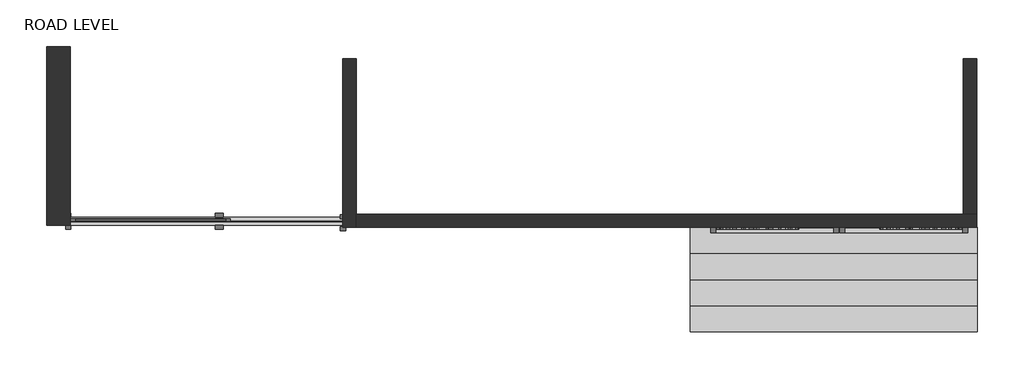
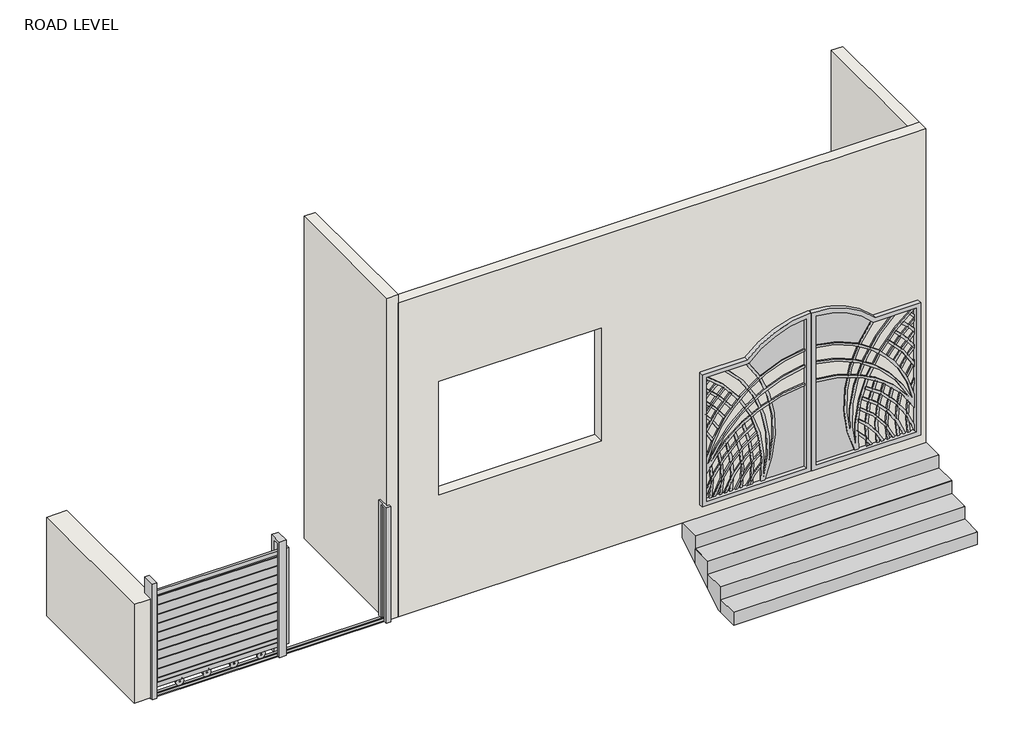
# One storey: 4 walls, 1 geographic element, 1 proxy, 1 stair flight.
"""IFC4 building model written with IfcOpenShell, lengths in millimetres."""

from ifc_helpers import new_model, si_unit, point, frame, frame_2d, origin, place, context, project, spatial, polyline, circle_curve, trimmed, segment, composite_curve, outline, extrude, faceted_brep, transform, mapped, element, save
from components import gate_7956_gate_7956_6bc30956

model = new_model("IFC4")

# Units and contexts
model_context = context("Model", 3, world=origin())
ifc_project = project(units=[si_unit("LENGTHUNIT", "METRE", prefix="MILLI")], contexts=[model_context])

# Site, building, storey
site = spatial("IfcSite", under=ifc_project)
building = spatial("IfcBuilding", under=site)
storey = spatial("IfcBuildingStorey", under=building, Name="ROAD LEVEL", Elevation=457.2)

# Proxy
placement = place(None, origin())
gate_7956_gate_7956_shape = gate_7956_gate_7956_6bc30956(model_context)
element("IfcBuildingElementProxy", 1, Name="gate_7956 : gate_7956", ObjectType="gate_7956 : gate_7956", at=placement, inside=storey, context=model_context, shape_type="MappedRepresentation", body=[
    mapped(gate_7956_gate_7956_shape, transform((8127.3305046, -8538.9053244, 1066.8), x_axis=(1.0, 0.0, 0.0), y_axis=(0.0, 1.0, 0.0), z_axis=(0.0, 0.0, 1.0))),
])

# Geographic element
element("IfcGeographicElement", 2, ObjectType="Sliding_Gate_17236 : Sliding_Gate_17236", at=placement, inside=storey, context=model_context, shape_type="SolidModel", body=[
    extrude(outline(polyline([(-8474.623372, 914.4), (-8443.6553244, 914.4), (-8443.6553244, 901.7), (-8519.8553244, 901.7), (-8519.8553244, 914.4), (-8489.076024, 914.4), (-8489.076024, 913.0780612), (-8474.623372, 913.0780612), (-8474.623372, 914.4)])), frame((742.1222446, 0.0, 0.0), z_axis=(1.0, 0.0, 0.0), x_axis=(0.0, 1.0, 0.0)), (0.0, 0.0, 1.0), 2649.5789518),
    faceted_brep([(792.9222446, -8405.5553244, 914.4), (792.9222446, -8443.6553244, 914.4), (788.1495839, -8443.6553244, 914.4), (788.1495839, -8405.5553244, 914.4), (792.9222446, -8443.6553244, 2260.6), (767.5222446, -8443.6553244, 2260.6), (767.5222446, -8443.6553244, 2089.1943747), (788.1495839, -8443.6553244, 2089.1943747), (767.5222446, -8519.8553244, 2260.6), (767.5222446, -8519.8553244, 2089.1943747), (792.9222446, -8519.8553244, 2260.6), (792.9222446, -8519.8553244, 914.4), (742.1222446, -8519.8553244, 914.4), (742.1222446, -8519.8553244, 2089.1943747), (742.1222446, -8557.9553244, 914.4), (792.9222446, -8557.9553244, 914.4), (792.9222446, -8557.9553244, 2286.0), (742.1222446, -8557.9553244, 2286.0), (742.1222446, -8405.5553244, 2286.0), (742.1222446, -8405.5553244, 2089.1943747), (792.9222446, -8405.5553244, 2286.0), (788.1495839, -8405.5553244, 2089.1943747)], [[[0, 1, 2, 3]], [[1, 4, 5, 6, 7, 2]], [[5, 8, 9, 6]], [[8, 10, 11, 12, 13, 9]], [[14, 15, 16, 17]], [[14, 17, 18, 19, 13, 12]], [[18, 20, 0, 3, 21, 19]], [[1, 0, 20, 16, 15, 11, 10, 4]], [[5, 4, 10, 8]], [[17, 16, 20, 18]], [[7, 21, 3, 2]], [[21, 7, 6, 9, 13, 19]], [[12, 11, 15, 14]]]),
    extrude(outline(polyline([(-8405.5553244, 2286.0), (-8405.5553244, 914.4), (-8443.6553244, 914.4), (-8443.6553244, 2247.9), (-8519.8553244, 2247.9), (-8519.8553244, 914.4), (-8557.9553244, 914.4), (-8557.9553244, 2286.0), (-8405.5553244, 2286.0)])), frame((2170.8722446, 0.0, 0.0), z_axis=(1.0, 0.0, 0.0), x_axis=(0.0, 1.0, 0.0)), (0.0, 0.0, 1.0), 76.2),
    extrude(outline(polyline([(2087.8280612, 2272.4722446), (2087.8280612, 837.3722446), (1033.7280612, 837.3722446), (1033.7280612, 2272.4722446), (2087.8280612, 2272.4722446)]), holes=[polyline([(2062.4280612, 862.7722446), (2062.4280612, 2247.0722446), (2056.0780612, 2247.0722446), (2056.0780612, 862.7722446), (2062.4280612, 862.7722446)]), polyline([(1954.4780612, 862.7722446), (1954.4780612, 2247.0722446), (1948.1280612, 2247.0722446), (1948.1280612, 862.7722446), (1954.4780612, 862.7722446)]), polyline([(1846.5280612, 862.7722446), (1846.5280612, 2247.0722446), (1840.1780612, 2247.0722446), (1840.1780612, 862.7722446), (1846.5280612, 862.7722446)]), polyline([(1738.5780612, 862.7722446), (1738.5780612, 2247.0722446), (1732.2280612, 2247.0722446), (1732.2280612, 862.7722446), (1738.5780612, 862.7722446)]), polyline([(1630.6280612, 862.7722446), (1630.6280612, 2247.0722446), (1624.2780612, 2247.0722446), (1624.2780612, 862.7722446), (1630.6280612, 862.7722446)]), polyline([(1522.6780612, 862.7722446), (1522.6780612, 2247.0722446), (1516.3280612, 2247.0722446), (1516.3280612, 862.7722446), (1522.6780612, 862.7722446)]), polyline([(1414.7280612, 862.7722446), (1414.7280612, 2247.0722446), (1408.3780612, 2247.0722446), (1408.3780612, 862.7722446), (1414.7280612, 862.7722446)]), polyline([(1306.7780612, 862.7722446), (1306.7780612, 2247.0722446), (1300.4280612, 2247.0722446), (1300.4280612, 862.7722446), (1306.7780612, 862.7722446)]), polyline([(1198.8280612, 862.7722446), (1198.8280612, 2247.0722446), (1192.4780612, 2247.0722446), (1192.4780612, 862.7722446), (1198.8280612, 862.7722446)]), polyline([(1090.8780612, 862.7722446), (1090.8780612, 2247.0722446), (1084.5280612, 2247.0722446), (1084.5280612, 862.7722446), (1090.8780612, 862.7722446)])]), frame((0.0, -8476.376024, 0.0), z_axis=(0.0, 1.0, 0.0), x_axis=(0.0, 0.0, 1.0)), (0.0, 0.0, 1.0), 12.7),
    extrude(outline(polyline([(2132.2780612, 2316.9222446), (2132.2780612, 792.9222446), (989.2780612, 792.9222446), (989.2780612, 2316.9222446), (2132.2780612, 2316.9222446)]), holes=[polyline([(2081.4780612, 843.7222446), (2081.4780612, 2266.1222446), (1040.0780612, 2266.1222446), (1040.0780612, 843.7222446), (2081.4780612, 843.7222446)])]), frame((0.0, -8482.726024, 0.0), z_axis=(0.0, 1.0, 0.0), x_axis=(0.0, 0.0, 1.0)), (0.0, 0.0, 1.0), 25.4),
    extrude(outline(composite_curve([segment(trimmed(circle_curve(frame_2d((957.5280612, 1402.5222446)), 44.45), [point((957.5280612, 1358.0722446))], [point((957.5280612, 1446.9722446))], False, "CARTESIAN"), True, "CONTINUOUS"), segment(trimmed(circle_curve(frame_2d((957.5280612, 1402.5222446)), 44.45), [point((957.5280612, 1446.9722446))], [point((957.5280612, 1358.0722446))], False, "CARTESIAN"), True, "CONTINUOUS")], self_intersect=False), holes=[composite_curve([segment(trimmed(circle_curve(frame_2d((957.5280612, 1402.5222446)), 6.35), [point((957.5280612, 1396.1722446))], [point((957.5280612, 1408.8722446))], True, "CARTESIAN"), True, "CONTINUOUS"), segment(trimmed(circle_curve(frame_2d((957.5280612, 1402.5222446)), 6.35), [point((957.5280612, 1408.8722446))], [point((957.5280612, 1396.1722446))], True, "CARTESIAN"), True, "CONTINUOUS")], self_intersect=False)]), frame((0.0, -8476.376024, 0.0), z_axis=(0.0, 1.0, 0.0), x_axis=(0.0, 0.0, 1.0)), (0.0, 0.0, 1.0), 12.7),
    extrude(outline(composite_curve([segment(trimmed(circle_curve(frame_2d((957.5280612, 2012.1222446)), 44.45), [point((957.5280612, 1967.6722446))], [point((957.5280612, 2056.5722446))], False, "CARTESIAN"), True, "CONTINUOUS"), segment(trimmed(circle_curve(frame_2d((957.5280612, 2012.1222446)), 44.45), [point((957.5280612, 2056.5722446))], [point((957.5280612, 1967.6722446))], False, "CARTESIAN"), True, "CONTINUOUS")], self_intersect=False), holes=[composite_curve([segment(trimmed(circle_curve(frame_2d((957.5280612, 2012.1222446)), 6.35), [point((957.5280612, 2005.7722446))], [point((957.5280612, 2018.4722446))], True, "CARTESIAN"), True, "CONTINUOUS"), segment(trimmed(circle_curve(frame_2d((957.5280612, 2012.1222446)), 6.35), [point((957.5280612, 2018.4722446))], [point((957.5280612, 2005.7722446))], True, "CARTESIAN"), True, "CONTINUOUS")], self_intersect=False)]), frame((0.0, -8476.376024, 0.0), z_axis=(0.0, 1.0, 0.0), x_axis=(0.0, 0.0, 1.0)), (0.0, 0.0, 1.0), 12.7),
    extrude(outline(composite_curve([segment(trimmed(circle_curve(frame_2d((957.5280612, 1707.3222446)), 44.45), [point((957.5280612, 1662.8722446))], [point((957.5280612, 1751.7722446))], False, "CARTESIAN"), True, "CONTINUOUS"), segment(trimmed(circle_curve(frame_2d((957.5280612, 1707.3222446)), 44.45), [point((957.5280612, 1751.7722446))], [point((957.5280612, 1662.8722446))], False, "CARTESIAN"), True, "CONTINUOUS")], self_intersect=False), holes=[composite_curve([segment(trimmed(circle_curve(frame_2d((957.5280612, 1707.3222446)), 6.35), [point((957.5280612, 1700.9722446))], [point((957.5280612, 1713.6722446))], True, "CARTESIAN"), True, "CONTINUOUS"), segment(trimmed(circle_curve(frame_2d((957.5280612, 1707.3222446)), 6.35), [point((957.5280612, 1713.6722446))], [point((957.5280612, 1700.9722446))], True, "CARTESIAN"), True, "CONTINUOUS")], self_intersect=False)]), frame((0.0, -8476.376024, 0.0), z_axis=(0.0, 1.0, 0.0), x_axis=(0.0, 0.0, 1.0)), (0.0, 0.0, 1.0), 12.7),
    extrude(outline(composite_curve([segment(trimmed(circle_curve(frame_2d((957.5280612, 1097.7222446)), 44.45), [point((957.5280612, 1053.2722446))], [point((957.5280612, 1142.1722446))], False, "CARTESIAN"), True, "CONTINUOUS"), segment(trimmed(circle_curve(frame_2d((957.5280612, 1097.7222446)), 44.45), [point((957.5280612, 1142.1722446))], [point((957.5280612, 1053.2722446))], False, "CARTESIAN"), True, "CONTINUOUS")], self_intersect=False), holes=[composite_curve([segment(trimmed(circle_curve(frame_2d((957.5280612, 1097.7222446)), 6.35), [point((957.5280612, 1091.3722446))], [point((957.5280612, 1104.0722446))], True, "CARTESIAN"), True, "CONTINUOUS"), segment(trimmed(circle_curve(frame_2d((957.5280612, 1097.7222446)), 6.35), [point((957.5280612, 1104.0722446))], [point((957.5280612, 1091.3722446))], True, "CARTESIAN"), True, "CONTINUOUS")], self_intersect=False)]), frame((0.0, -8476.376024, 0.0), z_axis=(0.0, 1.0, 0.0), x_axis=(0.0, 0.0, 1.0)), (0.0, 0.0, 1.0), 12.7),
    faceted_brep([(3366.3011964, -8418.2553244, 914.4), (3417.1011964, -8418.2553244, 914.4), (3417.1011964, -8570.6553244, 914.4), (3366.3011964, -8570.6553244, 914.4), (3366.3011964, -8532.5553244, 914.4), (3391.7011964, -8532.5553244, 914.4), (3391.7011964, -8456.3553244, 914.4), (3366.3011964, -8456.3553244, 914.4), (3391.7011964, -8456.3553244, 2260.6), (3366.3011964, -8456.3553244, 2260.6), (3391.7011964, -8532.5553244, 2260.6), (3366.3011964, -8532.5553244, 2260.6), (3366.3011964, -8570.6553244, 2286.0), (3417.1011964, -8570.6553244, 2286.0), (3417.1011964, -8418.2553244, 2286.0), (3366.3011964, -8418.2553244, 2286.0)], [[[0, 1, 2, 3, 4, 5, 6, 7]], [[6, 8, 9, 7]], [[5, 10, 8, 6]], [[4, 11, 10, 5]], [[12, 3, 2, 13]], [[13, 2, 1, 14]], [[14, 1, 0, 15]], [[11, 4, 3, 12, 15, 0, 7, 9]], [[9, 8, 10, 11]], [[12, 13, 14, 15]]]),
])

# Stair flight
element("IfcStairFlight", 3, ObjectType="1mm_Tread-150mm_Depth", at=placement, inside=storey, context=model_context, shape_type="SolidModel", body=[
    faceted_brep([(6712.3831457, -9288.9053244, 456.2), (6712.3831457, -9538.9053244, 456.2), (9454.4805046, -9538.9053244, 456.2), (9454.4805046, -9288.9053244, 456.2), (6712.3831457, -9288.9053244, 304.8), (6712.3831457, -9538.9053244, 304.8), (9454.4805046, -9538.9053244, 304.8), (9454.4805046, -9288.9053244, 304.8), (6712.3831457, -9038.9053244, 608.6), (6712.3831457, -9288.9053244, 608.6), (9454.4805046, -9288.9053244, 608.6), (9454.4805046, -9038.9053244, 608.6), (6712.3831457, -9038.9053244, 432.9262296), (6712.3831457, -9249.0861473, 304.8), (9454.4805046, -9249.0861473, 304.8), (9454.4805046, -9038.9053244, 432.9262296), (6712.3831457, -8788.9053244, 585.3262296), (6712.3831457, -8538.9053244, 737.7262296), (9454.4805046, -8538.9053244, 737.7262296), (9454.4805046, -8788.9053244, 585.3262296), (6712.3831457, -8788.9053244, 761.0), (6712.3831457, -9038.9053244, 761.0), (9454.4805046, -9038.9053244, 761.0), (9454.4805046, -8788.9053244, 761.0), (6712.3831457, -8538.9053244, 913.4), (6712.3831457, -8788.9053244, 913.4), (9454.4805046, -8788.9053244, 913.4), (9454.4805046, -8538.9053244, 913.4)], [[[0, 1, 2, 3]], [[1, 0, 4, 5]], [[2, 1, 5, 6]], [[3, 2, 6, 7]], [[8, 9, 10, 11]], [[4, 0, 9, 8, 12, 13]], [[0, 3, 10, 9]], [[3, 7, 14, 15, 11, 10]], [[5, 4, 13, 14, 7, 6]], [[14, 13, 12, 16, 17, 18, 19, 15]], [[20, 21, 22, 23]], [[21, 20, 16, 12, 8]], [[8, 11, 22, 21]], [[23, 22, 11, 15, 19]], [[24, 25, 26, 27]], [[25, 24, 17, 16, 20]], [[20, 23, 26, 25]], [[27, 26, 23, 19, 18]], [[24, 27, 18, 17]]]),
    extrude(outline(polyline([(6712.3831457, -9288.9053244), (9454.4805046, -9288.9053244), (9454.4805046, -9538.9053244), (6712.3831457, -9538.9053244), (6712.3831457, -9288.9053244)])), frame((0.0, 0.0, 456.2), z_axis=(0.0, 0.0, 1.0), x_axis=(1.0, 0.0, 0.0)), (0.0, 0.0, 1.0), 1.0),
    extrude(outline(polyline([(6712.3831457, -9038.9053244), (9454.4805046, -9038.9053244), (9454.4805046, -9288.9053244), (6712.3831457, -9288.9053244), (6712.3831457, -9038.9053244)])), frame((0.0, 0.0, 608.6), z_axis=(0.0, 0.0, 1.0), x_axis=(1.0, 0.0, 0.0)), (0.0, 0.0, 1.0), 1.0),
    extrude(outline(polyline([(6712.3831457, -8788.9053244), (9454.4805046, -8788.9053244), (9454.4805046, -9038.9053244), (6712.3831457, -9038.9053244), (6712.3831457, -8788.9053244)])), frame((0.0, 0.0, 761.0), z_axis=(0.0, 0.0, 1.0), x_axis=(1.0, 0.0, 0.0)), (0.0, 0.0, 1.0), 1.0),
    extrude(outline(polyline([(6712.3831457, -8538.9053244), (9454.4805046, -8538.9053244), (9454.4805046, -8788.9053244), (6712.3831457, -8788.9053244), (6712.3831457, -8538.9053244)])), frame((0.0, 0.0, 913.4), z_axis=(0.0, 0.0, 1.0), x_axis=(1.0, 0.0, 0.0)), (0.0, 0.0, 1.0), 1.0),
])

# Walls
element("IfcWall", 4, ObjectType="5\"", at=placement, inside=storey, context=model_context, shape_type="Brep", body=[
    faceted_brep([(3517.0722446, -8538.9053244, 914.4), (3517.0722446, -8411.9053244, 914.4), (3517.0722446, -6926.0053244, 914.4), (3517.0722446, -6926.0053244, 4749.8), (3517.0722446, -8538.9053244, 4749.8), (3517.0722446, -8538.9053244, 4648.2), (3390.0722446, -8538.9053244, 914.4), (3390.0722446, -8538.9053244, 4749.8), (3390.0722446, -6926.0053244, 4749.8), (3390.0722446, -6926.0053244, 2706.0311436), (3390.0722446, -6926.0053244, 914.4)], [[[0, 1, 2, 3, 4, 5]], [[6, 7, 8, 9, 10]], [[2, 1, 0, 6, 10]], [[4, 3, 8, 7]], [[0, 5, 4, 7, 6]], [[2, 10, 9, 8, 3]]]),
])
element("IfcWall", 5, ObjectType="5\"", at=placement, inside=storey, context=model_context, shape_type="Brep", body=[
    faceted_brep([(3517.0722446, -8538.9053244, 914.4), (9448.1305046, -8538.9053244, 914.4), (9448.1305046, -8538.9053244, 4648.2), (3517.0722446, -8538.9053244, 4648.2), (3974.2722446, -8538.9053244, 3555.2178666), (5803.0722446, -8538.9053244, 3555.2178666), (5803.0722446, -8538.9053244, 2209.0178666), (3974.2722446, -8538.9053244, 2209.0178666), (3517.0722446, -8411.9053244, 914.4), (3517.0722446, -8411.9053244, 4648.2), (9321.1305046, -8411.9053244, 4648.2), (9448.1305046, -8411.9053244, 4648.2), (9448.1305046, -8411.9053244, 914.4), (9321.1305046, -8411.9053244, 914.4), (3974.2722446, -8411.9053244, 3555.2178666), (3974.2722446, -8411.9053244, 2209.0178666), (5803.0722446, -8411.9053244, 2209.0178666), (5803.0722446, -8411.9053244, 3555.2178666)], [[[0, 1, 2, 3], [4, 5, 6, 7]], [[8, 9, 10, 11, 12, 13], [14, 15, 16, 17]], [[1, 0, 8, 13, 12]], [[3, 2, 11, 10, 9]], [[0, 3, 9, 8]], [[2, 1, 12, 11]], [[15, 14, 4, 7]], [[16, 15, 7, 6]], [[17, 16, 6, 5]], [[14, 17, 5, 4]]]),
])
element("IfcWall", 6, ObjectType="5\"", at=placement, inside=storey, context=model_context, shape_type="SweptSolid", body=[
    extrude(outline(polyline([(9448.1305046, -6926.0053244), (9448.1305046, -8411.9053244), (9321.1305046, -8411.9053244), (9321.1305046, -6926.0053244), (9448.1305046, -6926.0053244)])), frame((0.0, 0.0, 914.4), z_axis=(0.0, 0.0, 1.0), x_axis=(1.0, 0.0, 0.0)), (0.0, 0.0, 1.0), 3733.8),
])
element("IfcWall", 7, ObjectType="9\"", at=placement, inside=storey, context=model_context, shape_type="SweptSolid", body=[
    extrude(outline(polyline([(559.5495839, -8519.8553244), (559.5495839, -6811.7053244), (788.1495839, -6811.7053244), (788.1495839, -8519.8553244), (559.5495839, -8519.8553244)])), frame((0.0, 0.0, 914.4), z_axis=(0.0, 0.0, 1.0), x_axis=(1.0, 0.0, 0.0)), (0.0, 0.0, 1.0), 1174.7943747),
])

save(model, "model.ifc")

# Revit data of these elements
# Type "gate_7956 : gate_7956"
#   m.s. sheet = none
#   2" x2" pipe = none
#   1"x1"pipe = none
#   Default Elevation = 0
# Type "Sliding_Gate_17236 : Sliding_Gate_17236"
#   channel width = 10' - 0"
#   Width = 5' - 0"
#   Gate open = 0' - 0"
#   stopper material = aluminium dark grey
#   panel material = wood panel
# Type "5\""
#   Keynote = "F10"
#   Layers, outside or top first: 0' - 5" "Concrete" (function 1)
# Type "9\""
#   Keynote = "F10"
#   Layers, outside or top first: 0' - 9" "Concrete" (function 1)
# Element 1 (IfcBuildingElementProxy, "gate_7956 : gate_7956")
#   Phase Created = New Construction
#   Materials on its faces: "r1"
# Element 2 (IfcGeographicElement, "Sliding_Gate_17236 : Sliding_Gate_17236")
#   Phase Created = New Construction
#   Materials on its faces: "wood panel", "aluminium dark grey", "black metal"
# Element 3 (IfcStairFlight, "1mm_Tread-150mm_Depth")
#   Phase Created = New Construction
#   Materials on its faces: "Concrete, Cast-in-Place gray"
# Element 4 (IfcWall, "5\"")
#   built-in parameter 1001111 = 1' - 6"
#   Top Offset = 0' - 0"
#   Base Offset = 1' - 6"
#   Unconnected Height = 12' - 7"
#   wall height = 12' - 7"
#   Phase Created = New Construction
#   Base Constraint = ROAD LEVEL
#   Materials on its faces: "Concrete", "Gypsum Wall Board"
# Elements 5, 6 (IfcWall, "5\"")
#   built-in parameter 1001111 = 1' - 6"
#   Top Offset = 0' - 0"
#   Base Offset = 1' - 6"
#   Unconnected Height = 12' - 3"
#   wall height = 12' - 3"
#   Phase Created = New Construction
#   Base Constraint = ROAD LEVEL
#   Materials on its faces: "Concrete", "Gypsum Wall Board"
# Element 7 (IfcWall, "9\"")
#   built-in parameter 1001111 = 1' - 6"
#   Top Offset = 3' - 10.25175"
#   Base Offset = 1' - 6"
#   wall height = 3' - 10.25175"
#   Phase Created = New Construction
#   Base Constraint = ROAD LEVEL
#   Top Constraint = DRIVE LEV
#   Materials on its faces: "Concrete", "Gypsum Wall Board"
# Materials
#   "aluminium dark grey": class "Generic", colour RGB 85 85 85, transparency 0, Cost = 0
#   "wood panel": class "Generic", colour RGB 128 64 0, transparency 0, Cost = 0
#   "Concrete": class "Concrete", colour RGB 120 120 120, transparency 0, Description = "Portland Cement Concrete", Cost = 0
#   "r1": class "Generic", colour RGB 120 120 120, transparency 0, Cost = 0
#   "black metal": class "Generic", colour RGB 120 120 120, transparency 0, Cost = 0
#   "Concrete, Cast-in-Place gray": class "Concrete", colour RGB 192 192 192, transparency 0, Description = "Cast-in-place concrete", Cost = 0
#   "Gypsum Wall Board": class "Generic", colour RGB 249 249 249, transparency 0, Description = "Gypsum Wall Board", Cost = 0
